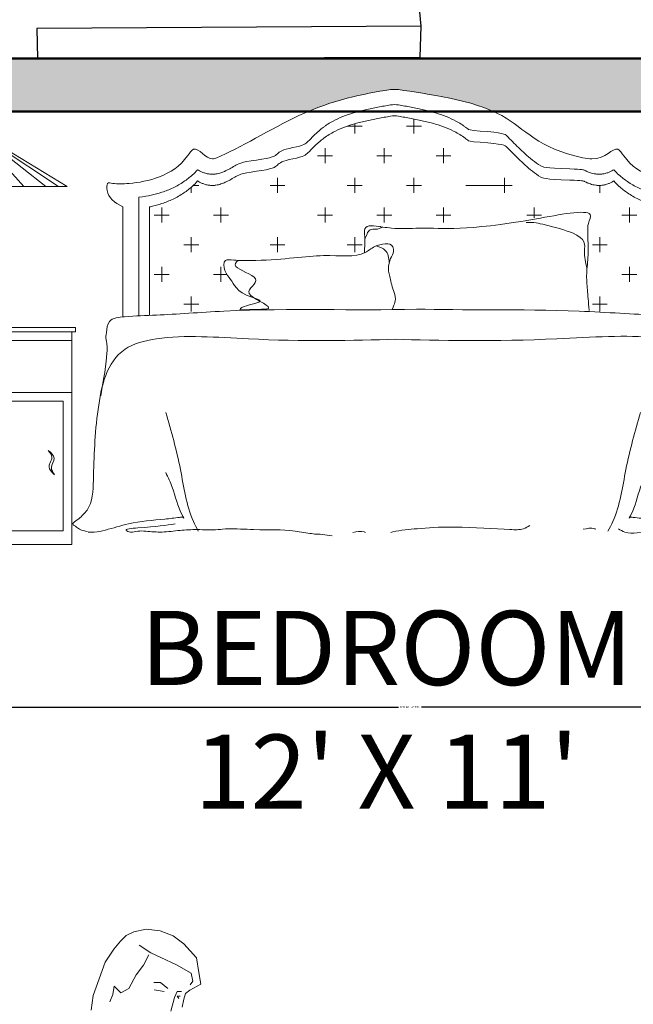
# Model space of a CAD drawing. Units: inches. Extents: x 1771 to 3025, y 319 to 889.
# Tile 4 of 35: x 1997 to 2055, y 527 to 620. Entities that reach past the tile are written whole.
import ezdxf

# ---------------------------------------------------------------- set-up
doc = ezdxf.new("R2010")
doc.units = ezdxf.units.IN
doc.header["$MEASUREMENT"] = 0
for name, color, linetype, lineweight in [('A-ANNO-DIMS', 2, 'Continuous', 18), ('A-AREA-IDEN', 241, 'Continuous', 25), ('A-DOOR', 4, 'Continuous', 25), ('A-FURN', 8, 'Continuous', 18), ('A-WALL', 7, 'Continuous', 50), ('A-WALL-PATT', 254, 'Continuous', 13)]:
    doc.layers.add(name, color=color, linetype=linetype, lineweight=lineweight)
doc.styles.get("Standard").update_dxf_attribs({"font": 'arial.ttf'})
doc.dimstyles.get("Standard").update_dxf_attribs({"dimtxt": 0.18, "dimasz": 0.18, "dimexe": 0.18, "dimexo": 0.0625, "dimgap": 0.09, "dimtad": 0, "dimtih": 1, "dimtoh": 1, "dimdec": 4, "dimzin": 0, "dimdsep": 46, "dimtxsty": 'Standard', "dimcen": 0.09, "dimadec": 0, "dimazin": 0, "dimtfac": 1, "dimtdec": 4, "dimtofl": 0, "dimtmove": 0, "dimatfit": 3, "dimfxl": 1, "dimtolj": 1, "dimtzin": 0, "dimarcsym": 0})

# ---------------------------------------------------------------- blocks, each defined once
blk = doc.blocks.new('A$C3908634B')
at = {"ltscale": 5}
for p, q in [((1200.2, 1046.3), (1218.1, 1046.3)), ((1176, 731), (1176, 731.7))]:
    blk.add_line(p, q, dxfattribs=at)
for p, q in [((1253.9, 945.1), (1253.9, 978.5)), ((1100.9, 962.2), (1134.6, 962.2)), ((1117.6, 945.1), (1117.6, 967.5)), ((1236.9, 962.2), (1271, 962.2)), ((266, 923.4), (356.4, 823.1)), ((278.7, 923.4), (406.8, 823.1)), ((284.7, 923.4), (436.3, 823.1)), ((290.6, 923.4), (456, 823.1)), ((1049.4, 876.9), (1049.4, 911)), ((1185.7, 876.9), (1185.7, 911)), ((1322.1, 876.9), (1322.1, 911)), ((1032.3, 894), (1066.4, 894)), ((1168.7, 894), (1202.8, 894)), ((1305.1, 894), (1339.1, 894)), ((940, 808.8), (940, 842.9)), ((1117.6, 808.8), (1117.6, 842.9)), ((1253.9, 808.8), (1253.9, 842.9)), ((1462.5, 808.8), (1462.5, 842.9)), ((237.5, 823.1), (456, 823.1)), ((741.7, 808.8), (741.7, 821.7)), ((746.2, 825.8), (758.8, 825.8)), ((922.9, 825.8), (957, 825.8)), ((1100.5, 825.8), (1134.6, 825.8)), ((1236.9, 825.8), (1271, 825.8)), ((1373.2, 825.8), (1479.5, 825.8)), ((1681.3, 808.8), (1681.3, 825.6)), ((621.3, 798.8), (621.3, 526)), ((645.8, 776.5), (645.8, 527)), ((673.5, 740.6), (673.5, 774.7)), ((809.9, 740.6), (809.9, 774.7)), ((1049.4, 740.6), (1049.4, 774.7)), ((1185.7, 740.6), (1185.7, 774.7)), ((1322.1, 740.6), (1322.1, 774.7)), ((1530.6, 751.3), (1530.6, 774.7)), ((1749.5, 740.6), (1749.5, 774.7)), ((656.5, 757.6), (690.6, 757.6)), ((792.9, 757.6), (827, 757.6)), ((1032.3, 757.6), (1066.4, 757.6)), ((1168.7, 757.6), (1202.8, 757.6)), ((1305.1, 757.6), (1339.1, 757.6)), ((1513.6, 757.6), (1547.7, 757.6)), ((1732.4, 757.6), (1766.5, 757.6)), ((741.7, 672.4), (741.7, 706.5)), ((940, 672.4), (940, 706.5)), ((1117.6, 672.4), (1117.6, 706.5)), ((1681.3, 672.4), (1681.3, 706.5)), ((724.7, 689.4), (758.8, 689.4)), ((922.9, 689.4), (957, 689.4)), ((1100.5, 689.4), (1134.6, 689.4)), ((1664.3, 689.4), (1698.3, 689.4)), ((673.5, 604.2), (673.5, 638.3)), ((809.9, 604.2), (809.9, 638.3)), ((1749.5, 604.2), (1749.5, 638.3)), ((656.5, 621.3), (690.6, 621.3)), ((792.9, 621.3), (823.2, 621.3)), ((1732.4, 621.3), (1766.5, 621.3)), ((741.7, 536), (741.7, 570.1)), ((1681.3, 536), (1681.3, 570.1)), ((724.7, 553.1), (758.8, 553.1)), ((1664.3, 553.1), (1698.3, 553.1)), ((475, 499.5), (0, 499.5)), ((475, 499.5), (475, 489.5)), ((475, 489.5), (0, 489.5)), ((467.1, 0), (467.1, 489.5)), ((467.1, 469.5), (8.7, 469.5)), ((467.1, 349.5), (8.7, 349.5)), ((447.1, 329.5), (28.7, 329.5)), ((447.1, 31.6), (447.1, 329.5)), ((467.1, 281.6), (467.1, 301.6)), ((28.7, 31.6), (447.1, 31.6)), ((8.7, 0), (467.1, 0))]:
    blk.add_line(p, q)
at = {"ltscale": 20}
blk.add_line((584.4, 776.7), (584.4, 523.7), dxfattribs=at)
for centre in [(1209.1, 956.2), (1209.1, 930.3)]:
    blk.add_arc(centre, 55.2, 80.5605, 99.4395)
for points in [[(584.4, 776.7), (563.9, 786.2), (546, 802.1), (547.3, 834.8), (564.5, 828.3), (620.6, 830.4), (706.4, 847.2), (752.1, 924.2), (778.1, 880.4), (846.1, 907.1), (1017.7, 1014.1), (1134.5, 1035.5), (1200.2, 1046.3)], [(1885.4, 776.7), (1905.9, 786.2), (1923.9, 802.1), (1922.5, 834.8), (1905.3, 828.3), (1849.2, 830.4), (1763.4, 847.2), (1717.7, 924.2), (1691.7, 880.4), (1541.2, 907.1), (1472.8, 1014.1), (1283.8, 1035.5), (1218.1, 1046.3)]]:
    blk.add_open_spline(points, degree=3, knots=[12.417853, 12.417853, 12.417853, 12.417853, 68.394536, 90.665986, 114.156853, 157.554067, 281.869614, 298.858744, 338.737111, 347.060176, 470.423438, 625.498764, 625.498764, 625.498764, 625.498764], dxfattribs=at)
for points, knots in [([(756.1, 861.8), (756.9, 861.3), (757.6, 860.9), (759.9, 859.6), (761.6, 858.7), (765.5, 856.8), (767.8, 855.8), (772.7, 854.1), (775.4, 853.3), (780.8, 852.2), (783.3, 851.8), (787.1, 851.6), (788.2, 851.5), (789.9, 851.5), (790.6, 851.5), (791.9, 851.5), (792.5, 851.5), (793.6, 851.6), (794.1, 851.6), (795.8, 851.8), (796.8, 851.9), (800.3, 852.3), (802.5, 852.8), (806.5, 853.8), (808.3, 854.3), (811.5, 855.4), (812.9, 855.9), (815.3, 856.9), (816.4, 857.4), (817.6, 857.9), (817.8, 858), (818.4, 858.2), (818.7, 858.4), (819.5, 858.7), (820, 859), (821.6, 859.7), (822.7, 860.2), (825.8, 861.7), (827.9, 862.8), (834, 866), (837.9, 868.3), (848.5, 874.9), (854.9, 879.4), (928.8, 888.8), (934.4, 893.5), (945, 903.2), (950, 908), (1000.9, 917.4), (1005.5, 922.1), (1014.4, 931), (1018.7, 935.3), (1027, 943.5), (1031.1, 947.3), (1036.9, 952.4), (1038.8, 954), (1042, 956.7), (1043.5, 957.9), (1045.8, 959.7), (1046.7, 960.3), (1048.5, 961.7), (1049.4, 962.3), (1052.1, 964.2), (1054, 965.5), (1059.7, 969.2), (1063.6, 971.5), (1074.8, 977.5), (1082.2, 980.9), (1098, 987.2), (1106.3, 990), (1123.7, 995.2), (1132.8, 997.5), (1151.5, 1001.8), (1161.1, 1003.8), (1180.5, 1007.4), (1190.2, 1009), (1200.1, 1010.7)], [328.6705, 328.6705, 328.6705, 328.6705, 329.609368, 329.609368, 331.487103, 331.487103, 333.620342, 333.620342, 335.753581, 335.753581, 337.507866, 337.507866, 338.182373, 338.182373, 338.607397, 338.607397, 338.959312, 338.959312, 339.311227, 339.311227, 340.015058, 340.015058, 341.722742, 341.722742, 343.430427, 343.430427, 345.138111, 345.138111, 346.845796, 346.845796, 347.37881, 347.37881, 347.911824, 347.911824, 348.977853, 348.977853, 351.109909, 351.109909, 355.374023, 355.374023, 363.902249, 363.902249, 379.258481, 379.258481, 394.614712, 394.614712, 409.970944, 409.970944, 425.327175, 425.327175, 440.683406, 440.683406, 456.039638, 456.039638, 463.285514, 463.285514, 469.01116, 469.01116, 472.593, 472.593, 476.17484, 476.17484, 483.338521, 483.338521, 497.665882, 497.665882, 522.309302, 522.309302, 546.952723, 546.952723, 571.596143, 571.596143, 596.239564, 596.239564, 619.876409, 619.876409, 619.876409, 619.876409]), ([(1713.7, 861.8), (1713, 861.3), (1712.2, 860.9), (1709.9, 859.6), (1708.2, 858.7), (1704.3, 856.8), (1702.1, 855.8), (1697.1, 854.1), (1694.4, 853.3), (1689.1, 852.2), (1686.5, 851.8), (1682.7, 851.6), (1681.7, 851.5), (1679.9, 851.5), (1679.2, 851.5), (1678, 851.5), (1677.4, 851.5), (1676.2, 851.6), (1675.7, 851.6), (1674.1, 851.8), (1673, 851.9), (1669.5, 852.3), (1667.3, 852.8), (1663.3, 853.8), (1661.5, 854.3), (1658.4, 855.4), (1657, 855.9), (1654.5, 856.9), (1653.4, 857.4), (1652.2, 857.9), (1652, 858), (1651.4, 858.2), (1651.2, 858.4), (1650.4, 858.7), (1649.8, 859), (1648.2, 859.7), (1647.1, 860.2), (1644, 861.7), (1641.9, 862.8), (1553.3, 866), (1549.4, 868.3), (1538.8, 874.9), (1532.4, 879.4), (1520.4, 888.8), (1514.8, 893.5), (1504.2, 903.2), (1499.2, 908), (1489.5, 917.4), (1484.9, 922.1), (1476.1, 931), (1471.8, 935.3), (1463.4, 943.5), (1459.4, 947.3), (1381.4, 952.4), (1379.5, 954), (1376.2, 956.7), (1374.8, 957.9), (1372.5, 959.7), (1371.6, 960.3), (1369.8, 961.7), (1368.9, 962.3), (1366.2, 964.2), (1364.3, 965.5), (1358.6, 969.2), (1354.6, 971.5), (1343.5, 977.5), (1336, 980.9), (1320.2, 987.2), (1311.9, 990), (1294.6, 995.2), (1285.5, 997.5), (1266.8, 1001.8), (1257.2, 1003.8), (1237.8, 1007.4), (1228.1, 1009), (1218.2, 1010.7)], [328.6705, 328.6705, 328.6705, 328.6705, 329.609368, 329.609368, 331.487103, 331.487103, 333.620342, 333.620342, 335.753581, 335.753581, 337.507866, 337.507866, 338.182373, 338.182373, 338.607397, 338.607397, 338.959312, 338.959312, 339.311227, 339.311227, 340.015058, 340.015058, 341.722742, 341.722742, 343.430427, 343.430427, 345.138111, 345.138111, 346.845796, 346.845796, 347.37881, 347.37881, 347.911824, 347.911824, 348.977853, 348.977853, 351.109909, 351.109909, 355.374023, 355.374023, 363.902249, 363.902249, 379.258481, 379.258481, 394.614712, 394.614712, 409.970943, 409.970943, 425.327175, 425.327175, 440.683406, 440.683406, 456.039637, 456.039637, 463.285514, 463.285514, 469.011154, 469.011154, 472.592992, 472.592992, 476.17483, 476.17483, 483.338506, 483.338506, 497.665857, 497.665857, 522.309275, 522.309275, 546.952693, 546.952693, 571.59611, 571.59611, 596.239528, 596.239528, 619.876409, 619.876409, 619.876409, 619.876409]), ([(756.1, 835.9), (756.9, 835.5), (757.6, 835), (759.9, 833.7), (761.6, 832.8), (765.5, 830.9), (767.8, 830), (772.7, 828.2), (775.4, 827.5), (780.8, 826.3), (783.3, 826), (787.1, 825.7), (788.2, 825.7), (789.9, 825.6), (790.6, 825.6), (791.9, 825.6), (792.5, 825.7), (793.6, 825.7), (794.1, 825.8), (795.8, 825.9), (796.8, 826), (800.3, 826.5), (802.5, 826.9), (806.5, 827.9), (808.3, 828.5), (811.5, 829.5), (812.9, 830.1), (815.3, 831), (816.4, 831.5), (817.6, 832), (817.8, 832.1), (818.4, 832.4), (818.7, 832.5), (819.5, 832.9), (820, 833.1), (821.6, 833.8), (822.7, 834.3), (825.8, 835.9), (827.9, 836.9), (834, 840.2), (837.9, 842.4), (848.5, 849), (854.9, 853.6), (928.8, 862.9), (934.4, 867.7), (945, 877.3), (950, 882.1), (1000.9, 891.6), (1005.5, 896.2), (1014.4, 905.2), (1018.7, 909.5), (1027, 917.6), (1031.1, 921.4), (1036.9, 926.6), (1038.8, 928.2), (1042, 930.9), (1043.5, 932), (1045.8, 933.8), (1046.7, 934.5), (1048.5, 935.8), (1049.4, 936.4), (1052.1, 938.4), (1054, 939.6), (1059.7, 943.3), (1063.6, 945.6), (1074.8, 951.6), (1082.2, 955), (1098, 961.3), (1106.3, 964.2), (1123.7, 969.3), (1132.8, 971.6), (1151.5, 975.9), (1161.1, 977.9), (1180.5, 981.5), (1190.2, 983.2), (1200.1, 984.8)], [328.6705, 328.6705, 328.6705, 328.6705, 329.609368, 329.609368, 331.487103, 331.487103, 333.620342, 333.620342, 335.753581, 335.753581, 337.507866, 337.507866, 338.182373, 338.182373, 338.607397, 338.607397, 338.959312, 338.959312, 339.311227, 339.311227, 340.015058, 340.015058, 341.722742, 341.722742, 343.430427, 343.430427, 345.138111, 345.138111, 346.845796, 346.845796, 347.37881, 347.37881, 347.911824, 347.911824, 348.977853, 348.977853, 351.109909, 351.109909, 355.374023, 355.374023, 363.902249, 363.902249, 379.258481, 379.258481, 394.614712, 394.614712, 409.970944, 409.970944, 425.327175, 425.327175, 440.683406, 440.683406, 456.039638, 456.039638, 463.285514, 463.285514, 469.01116, 469.01116, 472.593, 472.593, 476.17484, 476.17484, 483.338521, 483.338521, 497.665882, 497.665882, 522.309302, 522.309302, 546.952723, 546.952723, 571.596143, 571.596143, 596.239564, 596.239564, 619.876409, 619.876409, 619.876409, 619.876409]), ([(1713.7, 835.9), (1713, 835.5), (1712.2, 835), (1709.9, 833.7), (1708.2, 832.8), (1704.3, 830.9), (1702.1, 830), (1697.1, 828.2), (1694.4, 827.5), (1689.1, 826.3), (1686.5, 826), (1682.7, 825.7), (1681.7, 825.7), (1679.9, 825.6), (1679.2, 825.6), (1678, 825.6), (1677.4, 825.7), (1676.2, 825.7), (1675.7, 825.8), (1674.1, 825.9), (1673, 826), (1669.5, 826.5), (1667.3, 826.9), (1663.3, 827.9), (1661.5, 828.5), (1658.4, 829.5), (1657, 830.1), (1654.5, 831), (1653.4, 831.5), (1652.2, 832), (1652, 832.1), (1651.4, 832.4), (1651.2, 832.5), (1650.4, 832.9), (1649.8, 833.1), (1648.2, 833.8), (1647.1, 834.3), (1644, 835.9), (1641.9, 836.9), (1553.3, 840.2), (1549.4, 842.4), (1538.8, 849), (1532.4, 853.6), (1520.4, 862.9), (1514.8, 867.7), (1504.2, 877.3), (1499.2, 882.1), (1489.5, 891.6), (1484.9, 896.2), (1476.1, 905.2), (1471.8, 909.5), (1463.4, 917.6), (1459.4, 921.4), (1381.4, 926.6), (1379.5, 928.2), (1376.2, 930.9), (1374.8, 932), (1372.5, 933.8), (1371.6, 934.5), (1369.8, 935.8), (1368.9, 936.4), (1366.2, 938.4), (1364.3, 939.6), (1358.6, 943.3), (1354.6, 945.6), (1343.5, 951.6), (1336, 955), (1320.2, 961.3), (1311.9, 964.2), (1294.6, 969.3), (1285.5, 971.6), (1266.8, 975.9), (1257.2, 977.9), (1237.8, 981.5), (1228.1, 983.2), (1218.2, 984.8)], [328.6705, 328.6705, 328.6705, 328.6705, 329.609368, 329.609368, 331.487103, 331.487103, 333.620342, 333.620342, 335.753581, 335.753581, 337.507866, 337.507866, 338.182373, 338.182373, 338.607397, 338.607397, 338.959312, 338.959312, 339.311227, 339.311227, 340.015058, 340.015058, 341.722742, 341.722742, 343.430427, 343.430427, 345.138111, 345.138111, 346.845796, 346.845796, 347.37881, 347.37881, 347.911824, 347.911824, 348.977853, 348.977853, 351.109909, 351.109909, 355.374023, 355.374023, 363.902249, 363.902249, 379.258481, 379.258481, 394.614712, 394.614712, 409.970943, 409.970943, 425.327175, 425.327175, 440.683406, 440.683406, 456.039637, 456.039637, 463.285514, 463.285514, 469.011154, 469.011154, 472.592992, 472.592992, 476.17483, 476.17483, 483.338506, 483.338506, 497.665857, 497.665857, 522.309275, 522.309275, 546.952693, 546.952693, 571.59611, 571.59611, 596.239528, 596.239528, 619.876409, 619.876409, 619.876409, 619.876409]), ([(621.3, 798.8), (633.4, 799.9), (641.2, 801.3), (657.3, 805), (665.7, 807.2), (682.6, 812.8), (691.1, 816.1), (708.1, 824.2), (716.5, 828.9), (731.3, 839), (737.9, 844.1), (748.3, 853.5), (752.3, 857.5), (756.1, 861.8)], [179.330708, 179.330708, 179.330708, 179.330708, 196.086144, 196.086144, 213.445516, 213.445516, 230.804888, 230.804888, 248.16426, 248.16426, 262.451931, 262.451931, 271.832526, 271.832526, 271.832526, 271.832526]), ([(1848.6, 798.8), (1836.4, 799.9), (1828.6, 801.3), (1812.5, 805), (1804.1, 807.2), (1787.2, 812.8), (1778.7, 816.1), (1761.8, 824.2), (1753.4, 828.9), (1738.5, 839), (1731.9, 844.1), (1721.5, 853.5), (1717.5, 857.5), (1713.7, 861.8)], [179.400376, 179.400376, 179.400376, 179.400376, 196.086144, 196.086144, 213.445516, 213.445516, 230.804888, 230.804888, 248.16426, 248.16426, 262.451931, 262.451931, 271.832526, 271.832526, 271.832526, 271.832526]), ([(645.8, 776.5), (646.9, 776.7), (648, 777), (657.3, 779.1), (665.7, 781.3), (682.6, 786.9), (691.1, 790.3), (708.1, 798.3), (716.5, 803), (731.3, 813.1), (737.9, 818.2), (748.3, 827.7), (752.3, 831.7), (756.1, 835.9)], [193.740688, 193.740688, 193.740688, 193.740688, 196.086144, 196.086144, 213.445516, 213.445516, 230.804888, 230.804888, 248.16426, 248.16426, 262.451931, 262.451931, 271.832526, 271.832526, 271.832526, 271.832526]), ([(1824, 776.5), (1822.9, 776.7), (1821.8, 777), (1812.5, 779.1), (1804.1, 781.3), (1787.2, 786.9), (1778.7, 790.3), (1761.8, 798.3), (1753.4, 803), (1738.5, 813.1), (1731.9, 818.2), (1721.5, 827.7), (1717.5, 831.7), (1713.7, 835.9)], [193.740688, 193.740688, 193.740688, 193.740688, 196.086144, 196.086144, 213.445516, 213.445516, 230.804888, 230.804888, 248.16426, 248.16426, 262.451931, 262.451931, 271.832526, 271.832526, 271.832526, 271.832526]), ([(1181.8, 730.2), (1176.9, 727.3), (1167.9, 723.5), (1152.3, 726.4), (1145.2, 713.6), (1142.1, 705.5), (1140.6, 701.2)], [16.588235, 16.588235, 16.588235, 16.588235, 39.368234, 56.465167, 72.647278, 91.317886, 91.317886, 91.317886, 91.317886]), ([(1512.2, 740.7), (1519.9, 740.7), (1533.1, 740.8), (1553.9, 735.5), (1652.4, 710.7), (1643.1, 675.3), (1648.8, 648.1), (1651.8, 634.5), (1651.9, 634)], [0, 0, 0, 0, 31.268494, 53.71641, 83.24833, 138.583941, 192.96698, 194.695488, 194.695488, 194.695488, 194.695488]), ([(1167.2, 686.5), (1175.5, 684.3), (1192.8, 677.8), (1196.3, 659.6), (1197.1, 648.3)], [13.535772, 13.535772, 13.535772, 13.535772, 45.871957, 87.312392, 87.312392, 87.312392, 87.312392]), ([(849.2, 653.1), (844.3, 648.8), (832.7, 636.7), (919.4, 609.9), (841.8, 577.9), (927.1, 550.1), (918.1, 541), (854.7, 539.8)], [5.952535, 5.952535, 5.952535, 5.952535, 29.258845, 70.114919, 115.518645, 162.322231, 169.813565, 169.813565, 169.813565, 169.813565]), ([(412.3, 216.6), (419.2, 211), (432.8, 199.9), (414.9, 178.1), (423.4, 166), (427.2, 160.5)], [0, 0, 0, 0, 22.772447, 45.052082, 63.466582, 63.466582, 63.466582, 63.466582]), ([(412.3, 216.6), (416.7, 211.4), (424.6, 201.9), (416.9, 189), (411.8, 174.1), (420.6, 166.3), (427.2, 160.5)], [0, 0, 0, 0, 18.381528, 32.980054, 40.875646, 63.595153, 63.595153, 63.595153, 63.595153])]:
    blk.add_open_spline(points, degree=3, knots=knots)
at = {"ltscale": 5}
for points, knots in [([(1140.2, 671), (1140.5, 684.2), (1141, 702.6), (1139.6, 733.3), (1171.5, 732.8), (1207.8, 724.4), (1313, 731.7), (1377.9, 716.1), (1675.3, 776), (1653.6, 739.3), (1653.4, 708.6), (1656.7, 669.4), (1649.8, 624.8), (1652.8, 584.9), (1655.4, 559.2), (1656.8, 538.3)], [3.603347, 3.603347, 3.603347, 3.603347, 60.838375, 82.182907, 107.012175, 163.177093, 249.239778, 501.114283, 577.787612, 607.274607, 630.949286, 706.159707, 762.92633, 812.910096, 867.096105, 867.096105, 867.096105, 867.096105]), ([(853.1, 539.8), (853.8, 547.4), (919.3, 558.2), (845.3, 575.8), (836.7, 609.7), (818, 623.2), (814.4, 657.6), (840.5, 653), (943.6, 652.6), (1051.1, 671.7), (1127.7, 657.4), (1165, 689.4), (1205, 697), (1208.2, 671.1), (1198.6, 657.5), (1193.8, 634.4), (1197.9, 619.2), (1201.2, 597.1), (1215.4, 563.6), (1206.8, 549.2), (1203.5, 540.2)], [33.020195, 33.020195, 33.020195, 33.020195, 57.294753, 90.473933, 194.149416, 257.058105, 304.592565, 338.383824, 389.043604, 577.649845, 759.359611, 813.032269, 898.973184, 920.659088, 956.429806, 1000.911745, 1042.797508, 1121.842246, 1191.460876, 1213.109701, 1213.109701, 1213.109701, 1213.109701]), ([(533.2, 342.2), (554.6, 456.3), (543.3, 464.8), (546.8, 491.4), (549.9, 520.4), (602.8, 525.9), (675.3, 527.2), (929.2, 547.1), (1113.3, 536.9), (1259.7, 541.4)], [0, 0, 0, 0, 32.681627, 48.455722, 75.25348, 112.004017, 183.381957, 310.642358, 688.088714, 688.088714, 688.088714, 688.088714]), ([(1911, 390.4), (1911.9, 458.8), (1930, 464.8), (1926.5, 491.4), (1923.4, 520.4), (1870.5, 525.9), (1798, 527.2), (1556.5, 543.7), (1364.8, 538.4), (1259.7, 541.4)], [0, 0, 0, 0, 32.681627, 48.455722, 75.25348, 112.004017, 183.381957, 310.642358, 588.939547, 588.939547, 588.939547, 588.939547]), ([(482.8, 59.4), (489.8, 65.8), (514.7, 88.6), (517.4, 182.5), (520.5, 297.5), (551.9, 447.1), (697, 485.5), (926.3, 465.8), (1116.6, 468.9), (1210.9, 472.2)], [0, 0, 0, 0, 28.320233, 100.953775, 269.820348, 420.691469, 489.161544, 656.134073, 940.569207, 940.569207, 940.569207, 940.569207]), ([(1990.5, 59.4), (1983.5, 65.8), (1958.6, 88.6), (1942.6, 182.5), (1920.4, 297.5), (1912.1, 455.6), (1776.3, 485.5), (1526.4, 465.8), (1305.2, 468.9), (1210.9, 472.2)], [0, 0, 0, 0, 28.320233, 100.953775, 269.820348, 420.691469, 489.161544, 656.134073, 940.569207, 940.569207, 940.569207, 940.569207]), ([(682.9, 304.1), (695.4, 260.8), (719.1, 178.1), (730.8, 82.2), (753.9, 38.3), (757.8, 30.9)], [0, 0, 0, 0, 135.247847, 258.692787, 283.800228, 283.800228, 283.800228, 283.800228]), ([(1775.2, 304.1), (1762.7, 260.8), (1739, 178.1), (1727.3, 82.2), (1704.2, 38.3), (1700.3, 30.9)], [0, 0, 0, 0, 135.247847, 258.692787, 283.800228, 283.800228, 283.800228, 283.800228]), ([(682.9, 165.6), (688.3, 154.5), (703.5, 123.2), (710.2, 85), (723.1, 63.5), (724.6, 61.1)], [0, 0, 0, 0, 37.234018, 105.386078, 113.844905, 113.844905, 113.844905, 113.844905]), ([(1790.4, 165.6), (1785, 154.5), (1769.8, 123.2), (1763.1, 85), (1750.2, 63.5), (1748.7, 61.1)], [0, 0, 0, 0, 37.234018, 105.386078, 113.844905, 113.844905, 113.844905, 113.844905]), ([(482.8, 59.4), (474.7, 54.3), (464, 47.4), (477.3, 41.4), (486.1, 33.4), (496.5, 31.3), (502.9, 30)], [0, 0, 0, 0, 19.035414, 25.269998, 36.960672, 56.00812, 56.00812, 56.00812, 56.00812]), ([(504.2, 28.9), (509, 28.7), (522.4, 28.3), (553.7, 35.4), (605.7, 52.4), (665.1, 57), (705.3, 61.4), (721.5, 63.6), (724.2, 61.4), (724.6, 61.1)], [0, 0, 0, 0, 14.447875, 40.468341, 96.220884, 181.018327, 216.046098, 224.609189, 226.185962, 226.185962, 226.185962, 226.185962]), ([(704.5, 47.7), (683.7, 44.6), (656.6, 40.6), (582.3, 36), (604.8, 26.7), (618.5, 32.3), (643.5, 30.4), (675.7, 27.4), (715, 33.3), (758.1, 35.6), (793.8, 32.4), (824.3, 37.8), (918.5, 32.1), (952.2, 36.4), (1023, 23.8), (1044.1, 24.1), (1058.3, 21.3), (1065.7, 20.4)], [0, 0, 0, 0, 87.513803, 114.592793, 124.77702, 141.903576, 160.817021, 198.691115, 240.471478, 280.23486, 329.410006, 348.41762, 373.077233, 428.05708, 447.802257, 468.691939, 491.310217, 491.310217, 491.310217, 491.310217]), ([(1969.1, 28.9), (1964.3, 28.7), (1950.9, 28.3), (1919.6, 35.4), (1867.6, 52.4), (1808.2, 57), (1768, 61.4), (1751.8, 63.6), (1749.1, 61.4), (1748.7, 61.1)], [0, 0, 0, 0, 14.447875, 40.468341, 96.220884, 181.018327, 216.046098, 224.609189, 226.185962, 226.185962, 226.185962, 226.185962]), ([(1113.3, 28), (1122.2, 29.4), (1132.2, 31.9), (1141.4, 28.4), (1142.4, 28)], [516.212662, 516.212662, 516.212662, 516.212662, 542.681017, 546.007116, 546.007116, 546.007116, 546.007116]), ([(1200.5, 28), (1202, 28.4), (1222.7, 33.5), (1266.3, 36.8), (1334.2, 43.2), (1462.5, 35), (1502.7, 33.5), (1515.8, 41.2), (1520.7, 44.1)], [590.079786, 590.079786, 590.079786, 590.079786, 594.646549, 651.888327, 725.747367, 797.841373, 826.274406, 843.189267, 843.189267, 843.189267, 843.189267]), ([(1643.2, 35.6), (1652.1, 37), (1662.2, 39.5), (1671.4, 36), (1672.4, 35.6)], [516.212662, 516.212662, 516.212662, 516.212662, 542.681017, 546.007116, 546.007116, 546.007116, 546.007116]), ([(1972.3, 20.4), (1970.7, 20.8), (1950, 25.9), (1906.5, 29.2), (1838.6, 35.6), (1782.4, 27.4), (1742.2, 25.9), (1729.1, 33.6), (1724.3, 36.5)], [590.079786, 590.079786, 590.079786, 590.079786, 594.646549, 651.888327, 725.747367, 797.841373, 826.274406, 843.189267, 843.189267, 843.189267, 843.189267])]:
    blk.add_open_spline(points, degree=3, knots=knots, dxfattribs=at)
blk = doc.blocks.new('A$C0DCF6C46')
for p, q in [((1227.6, 1090.4), (1251, 1095.4)), ((1227.6, 1090.4), (1251, 1095.4)), ((1251, 1095.4), (1277.5, 1092)), ((1251, 1095.4), (1277.5, 1092)), ((1202.6, 1072.4), (1213.4, 1083.3)), ((1202.6, 1072.4), (1213.4, 1083.3)), ((1213.4, 1083.3), (1227.6, 1090.4)), ((1213.4, 1083.3), (1227.6, 1090.4)), ((1277.5, 1092), (1301.8, 1082.8)), ((1277.5, 1092), (1301.8, 1082.8)), ((1301.8, 1082.8), (1321.9, 1067.8)), ((1301.8, 1082.8), (1321.9, 1067.8)), ((1173.6, 1032.9), (1189.7, 1057.2)), ((1173.6, 1032.9), (1189.7, 1057.2)), ((1189.7, 1057.2), (1202.6, 1072.4)), ((1189.7, 1057.2), (1202.6, 1072.4)), ((1259.7, 1050.3), (1237.5, 1065.3)), ((1259.7, 1050.3), (1237.5, 1065.3)), ((1321.9, 1067.8), (1345.5, 1041.1)), ((1321.9, 1067.8), (1345.5, 1041.1)), ((1255.9, 1046.6), (1245.7, 1027.6)), ((1255.9, 1046.6), (1245.7, 1027.6)), ((1278.7, 1041.6), (1259.7, 1050.3)), ((1278.7, 1041.6), (1259.7, 1050.3)), ((1308.3, 1028.1), (1278.7, 1041.6)), ((1308.3, 1028.1), (1278.7, 1041.6)), ((1345.5, 1041.1), (1350.1, 1013.5)), ((1345.5, 1041.1), (1350.1, 1013.5)), ((1150.8, 970.5), (1173.6, 1032.9)), ((1150.8, 970.5), (1173.6, 1032.9)), ((1245.7, 1027.6), (1232.3, 1009.1)), ((1245.7, 1027.6), (1232.3, 1009.1)), ((1335.8, 1012.5), (1308.3, 1028.1)), ((1335.8, 1012.5), (1308.3, 1028.1)), ((1232.3, 1009.1), (1218.3, 983.7)), ((1232.3, 1009.1), (1218.3, 983.7)), ((1338.8, 997.1), (1335.8, 1012.5)), ((1338.8, 997.1), (1335.8, 1012.5)), ((1350.1, 1013.5), (1354.2, 991.7)), ((1350.1, 1013.5), (1354.2, 991.7)), ((1190.8, 987.7), (1188, 972.3)), ((1190.8, 987.7), (1188, 972.3)), ((1202.9, 975.4), (1190.8, 987.7)), ((1202.9, 975.4), (1190.8, 987.7)), ((1218.3, 983.7), (1202.9, 975.4)), ((1218.3, 983.7), (1202.9, 975.4)), ((1277.8, 994.4), (1265.6, 995)), ((1277.8, 994.4), (1265.6, 995)), ((1291.5, 983.2), (1277.8, 994.4)), ((1291.5, 983.2), (1277.8, 994.4)), ((1354.2, 991.7), (1333.4, 980.2)), ((1354.2, 991.7), (1333.4, 980.2)), ((1334, 990.3), (1338.8, 997.1)), ((1334, 990.3), (1338.8, 997.1)), ((1147.4, 942.9), (1150.8, 970.5)), ((1147.4, 942.9), (1150.8, 970.5)), ((1188, 972.3), (1182.6, 958)), ((1188, 972.3), (1182.6, 958)), ((1266, 980.7), (1284.6, 977.9)), ((1266, 980.7), (1284.6, 977.9)), ((1304.1, 966.6), (1297.6, 940.6)), ((1304.1, 966.6), (1297.6, 940.6)), ((1309.5, 977.7), (1304.1, 966.6)), ((1309.5, 977.7), (1304.1, 966.6)), ((1309.4, 969), (1312.6, 964.7)), ((1314.7, 968.9), (1309.4, 969)), ((1309.4, 969), (1312.6, 964.7)), ((1314.7, 968.9), (1309.4, 969)), ((1317.5, 977.7), (1309.5, 977.7)), ((1317.5, 977.7), (1309.5, 977.7)), ((1324.9, 973.9), (1322.1, 963.3)), ((1324.9, 973.9), (1322.1, 963.3)), ((1333.4, 980.2), (1324.9, 973.9)), ((1333.4, 980.2), (1324.9, 973.9)), ((1322.1, 963.3), (1318.8, 948.5)), ((1322.1, 963.3), (1318.8, 948.5))]:
    blk.add_line(p, q)
blk = doc.blocks.new('A$C4223307F')
blk.add_blockref('A$C0DCF6C46', (0, 0))
blk = doc.blocks.new('A$C061F63B6')
blk.add_blockref('A$C4223307F', (0, 0))
blk = doc.blocks.new('DOOR-35')
blk.add_lwpolyline([(35.881, 36.185), (32.957, 36.297), (33.165, 0), (36, 0.055)], close=True)
blk.add_arc((35.225, 1.111), 35.259, 93.68792, 177.49253)
blk = doc.blocks.new('*D40')
at = {"layer": 'A-ANNO-DIMS', "color": 0, "lineweight": -2, "transparency": 16777216}
for p, q in [((1983.209, 570.711), (1983.209, 555.266)), ((2085.389, 570.711), (2085.389, 555.266)), ((1983.389, 555.446), (2033.223, 555.446)), ((2085.209, 555.446), (2035.375, 555.446))]:
    blk.add_line(p, q, dxfattribs=at)
at = {"layer": 'A-ANNO-DIMS', "color": 0, "transparency": 16777216}
for points in [[(1983.389, 555.476), (1983.389, 555.416), (1983.209, 555.446)], [(2085.209, 555.476), (2085.209, 555.416), (2085.389, 555.446)]]:
    blk.add_solid(points, dxfattribs=at)
at = {"layer": 'Defpoints', "color": 0, "transparency": 16777216}
for p in [(1983.209, 570.773), (2085.389, 570.773), (2085.389, 555.446)]:
    blk.add_point(p, dxfattribs=at)
at = {"layer": 'A-ANNO-DIMS', "color": 0, "transparency": 16777216, "insert": (2034.299, 555.446), "char_height": 0.18, "attachment_point": 5}
blk.add_mtext('\\A1;BED B2 102 TYP.', dxfattribs=at)

msp = doc.modelspace()

# ---------------------------------------------------------------- hatches: boundary and pattern name
at = {"layer": 'A-WALL-PATT'}
h = msp.add_hatch(color=256, dxfattribs=at)
h.dxf.hatch_style = 1
h.paths.add_polyline_path([(1870.724, 888.634), (1799.724, 888.634), (1799.724, 878.634), (1870.724, 878.634)])
h.paths.add_polyline_path([(1968.767, 888.634), (1918.724, 888.634), (1918.724, 878.634), (1941.724, 878.634), (1941.724, 830.634), (1946.724, 830.634), (1946.724, 878.634), (1968.767, 878.634)])
h.paths.add_polyline_path([(2059.676, 888.634), (2016.767, 888.634), (2016.767, 878.634), (2037.724, 878.634), (2037.724, 794.634), (1941.724, 794.634), (1941.724, 758.634), (1941.724, 664.634), (1946.724, 664.634), (1946.724, 712), (1946.724, 789.634), (2054.724, 789.634), (2054.724, 794.634), (2042.325, 794.634), (2042.325, 798.62), (2042.325, 835.497), (2042.724, 878.634), (2059.676, 878.634)])
h.paths.add_polyline_path([(2100.724, 888.634), (2077.676, 888.634), (2077.676, 878.634), (2090.724, 878.634), (2090.724, 789.634), (2090.724, 768.608), (2100.724, 768.608)])
h.paths.add_polyline_path([(2100.724, 720.608), (2090.724, 720.608), (2090.724, 669.634), (1982.724, 669.634), (1982.724, 664.634), (2001.724, 664.634), (2001.724, 652.634), (2006.724, 652.634), (2006.724, 664.634), (2049.518, 664.634, -0.385549), (2050.522, 664.634), (2090.724, 664.634), (2090.724, 649.173), (2100.724, 649.173)])
edge = h.paths.add_edge_path()
edge.add_line((2100.724, 631.173), (2090.724, 631.173))
edge.add_line((2090.724, 631.173), (2090.724, 616.634))
edge.add_line((2090.724, 616.634), (2001.724, 616.634))
edge.add_line((2001.724, 616.634), (1982.724, 616.634))
edge.add_line((1982.724, 616.634), (1982.724, 611.634))
edge.add_line((1982.724, 611.634), (2024.672, 611.634))
edge.add_spline(control_points=[(2024.672, 611.634), (2027.581, 612.871), (2030.014, 613.313), (2032.469, 613.716)], knot_values=[484.321569, 484.321569, 484.321569, 484.321569, 625.498764, 625.498764, 625.498764, 625.498764], degree=3, periodic=0)
edge.add_line((2032.469, 613.716), (2033.205, 613.716))
edge.add_spline(control_points=[(2033.205, 613.716), (2035.66, 613.313), (2039.461, 612.871), (2042.204, 611.634)], knot_values=[484.321569, 484.321569, 484.321569, 484.321569, 625.498764, 625.498764, 625.498764, 625.498764], degree=3, periodic=0)
edge.add_line((2042.204, 611.634), (2090.724, 611.634))
edge.add_line((2090.724, 611.634), (2090.724, 581.106))
edge.add_line((2090.724, 581.106), (2100.724, 581.106))
edge.add_line((2100.724, 581.106), (2100.724, 631.173))
h.paths.add_polyline_path([(2100.724, 533.106), (2090.724, 533.106), (2090.724, 479.634), (1946.724, 479.634), (1946.724, 616.634), (1936.724, 616.634), (1936.724, 543.634), (1845.724, 543.634), (1845.724, 533.634), (1936.724, 533.634), (1936.724, 469.634), (2090.724, 469.634), (2090.724, 452.762), (2100.724, 452.762)])
h.paths.add_polyline_path([(2100.724, 404.762), (2090.724, 404.762), (2090.724, 393.634), (1936.724, 393.634), (1936.724, 383.634), (2100.724, 383.634)])
h.paths.add_polyline_path([(1905.724, 758.634), (1835.47, 758.634), (1835.47, 758.634), (1813.444, 758.634), (1809.724, 758.634), (1809.724, 842.589, -0.008336), (1808.421, 842.634), (1799.724, 842.634), (1799.724, 690.584), (1809.724, 690.584), (1809.724, 753.634), (1905.724, 753.634)])
h.paths.add_polyline_path([(1809.724, 642.584), (1799.724, 642.584), (1799.724, 533.634), (1809.724, 533.634), (1809.724, 581)])

# ---------------------------------------------------------------- linework, layer by layer
at = {"layer": 'A-WALL'}
for p, q in [((2001.724, 616.634), (1982.724, 616.634)), ((2090.724, 616.634), (2001.724, 616.634)), ((2090.724, 611.634), (1982.724, 611.634))]:
    msp.add_line(p, q, dxfattribs=at)

# ---------------------------------------------------------------- block references
at = {"layer": 'A-DOOR', "rotation": 269.9999999999959}
msp.add_blockref('DOOR-35', (1999.062, 652.634), dxfattribs=at)
at = {"layer": 'A-FURN'}
for name, p, xscale, yscale, zscale in [('A$C3908634B', (1983.209, 570.773), 0.0410441893854556, 0.0410441893854556, 0.0410441893854556), ('A$C061F63B6', (1946.724, 479.634), 0.0500958271542837, 0.0500958271542837, 0.0500958271542837)]:
    msp.add_blockref(name, p, dxfattribs=dict(at, xscale=xscale, yscale=yscale, zscale=zscale))

# ---------------------------------------------------------------- texts
at = {"layer": 'A-AREA-IDEN', "insert": (1989.356, 564.529), "char_height": 7, "attachment_point": 1}
msp.add_mtext_dynamic_manual_height_columns("\\pxqc;BEDROOM\\P12' X 11'", width=85.46108, gutter_width=1, heights=[0], dxfattribs=at)

# ---------------------------------------------------------------- dimensions: what is measured, and where the dimension line sits
at = {"layer": 'A-ANNO-DIMS'}
dim = msp.add_linear_dim(base=(2085.389, 555.446), p1=(1983.209, 570.773), p2=(2085.389, 570.773), text='BED B2 <> TYP.', dimstyle='Standard', override={"dimdec": 0, "dimrnd": 0, "dimzin": 0, "dimlunit": 2}, dxfattribs=at)
dim.commit()
dim.dimension.update_dxf_attribs({"geometry": '*D40', "text_midpoint": (2034.299, 555.446)})

doc.saveas('drawing.dxf')
